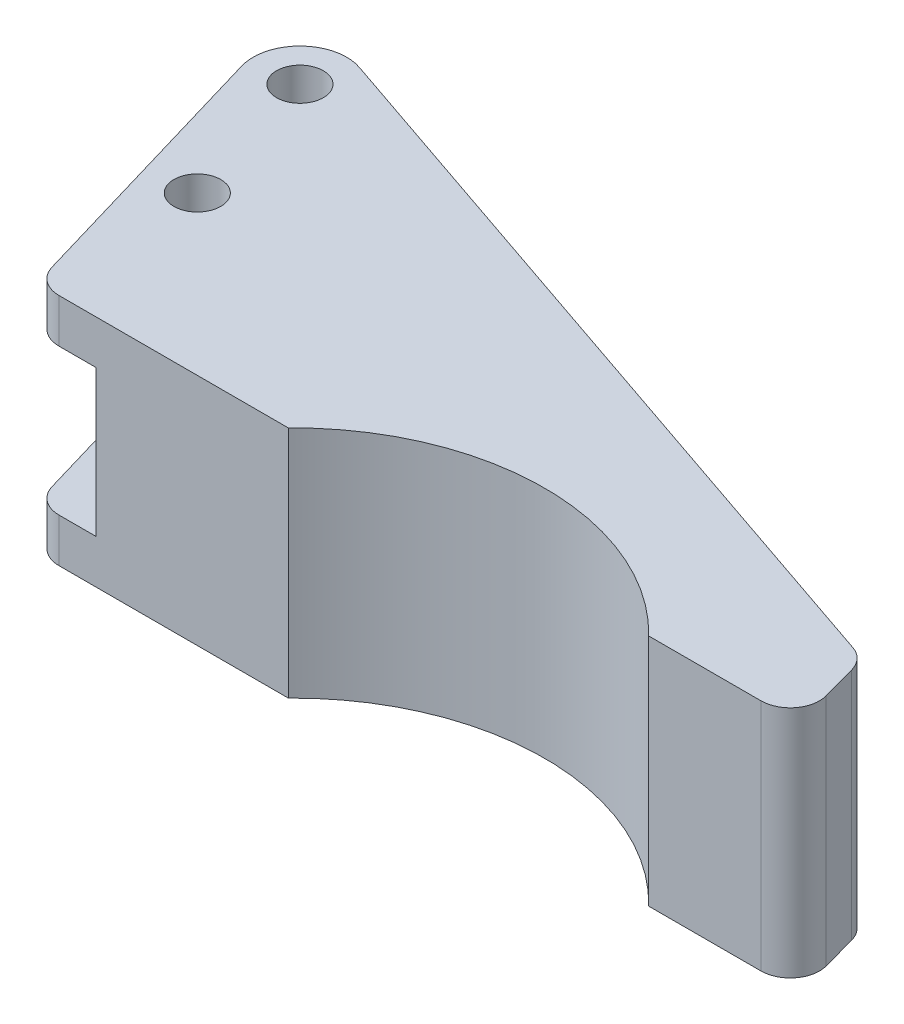
SolidWorks part; units mm, degrees
material "Plain Carbon Steel"
ref_plane "Front Plane" through (0, 0, 0) normal (0, 0, 1) x (1, 0, 0)
ref_plane "Top Plane" through (0, 0, 0) normal (0, 1, 0) x (1, 0, 0)
ref_plane "Right Plane" through (0, 0, 0) normal (1, 0, 0) x (0, 0, -1)
sketch "Bracket Profile Sketch" plane through (0, 0, 0) normal (0, 1, 0) x (1, 0, 0)
  line L0 (-1000, 0) -> (49000, 0) construction
  line L1 (0, -1000) -> (0, 49000) construction
  line L2 (-1.0572, 3.5861) -> (-14.6248, 49.6078)
  line L3 (-4.3673, 59.4412) -> (123.7037, 15.732)
  line L4 (126.9097, 12.3258) -> (128.5597, 6.3258)
  line L5 (123.7387, 0) -> (104.5446, 0)
  line L6 (42.9329, 0) -> (3.7387, 0)
  arc A0 (104.5446, 0) -> (42.9329, 0) centre (73.7387, -30) ccw
  arc A1 (-4.3673, 59.4412) -> (-14.6248, 49.6078) centre (-6.9513, 51.87) ccw
  arc A2 (126.9097, 12.3258) -> (123.7037, 15.732) centre (122.0887, 11) ccw
  arc A3 (128.5597, 6.3258) -> (123.7387, 0) centre (123.7387, 5) cw
  arc A4 (-1.0572, 3.5861) -> (3.7387, 0) centre (3.7387, 5) ccw
  point P22 (130.2993, 0)
  point P25 (0, 0)
  dimension "D1" = 8
  dimension "D2" = 5
  dimension "D3" = 43
  dimension "D4" = 30
  dimension "D5" = 70
  dimension "D6" = 120
  dimension "D7" = 51.87
  dimension "D8" = 10.69
  dimension "D9" = 6
  dimension "D10" = 1.65
extrude "Bracket Body" add sketch "Bracket Profile Sketch" along normal mid plane 40
sketch "Mounting Holes Sketch" plane through (0, 0, 0) normal (0, 1, 0) x (1, 0, 0)
  circle A0 centre (-6.9513, 51.87) radius 4
  circle A1 centre (0.3787, 27) radius 4
  dimension "D1" = 8
  dimension "D2" = 8
  dimension "D3" = 7.33
  dimension "D4" = 24.87
extrude "Mounting Holes 2xØ8" cut sketch "Mounting Holes Sketch" against normal mid plane 40
sketch "End Slot Sketch" plane through (0, 0, 0) normal (0, 0, 1) x (1, 0, 0)
  line L1 (-14.9513, 12.5) -> (10.0487, 12.5)
  line L2 (-14.9513, 12.5) -> (-14.9513, -12.5)
  line L3 (-14.9513, -12.5) -> (10.0487, -12.5)
  line L4 (10.0487, 12.5) -> (10.0487, -12.5)
  line L5 (-14.9513, 20) -> (-14.9513, -20) construction
  dimension "D1" = 25
  dimension "D2" = 25
  dimension "D3" = 12.5
extrude "End Slot 25 Wide" cut sketch "End Slot Sketch" against normal through all
